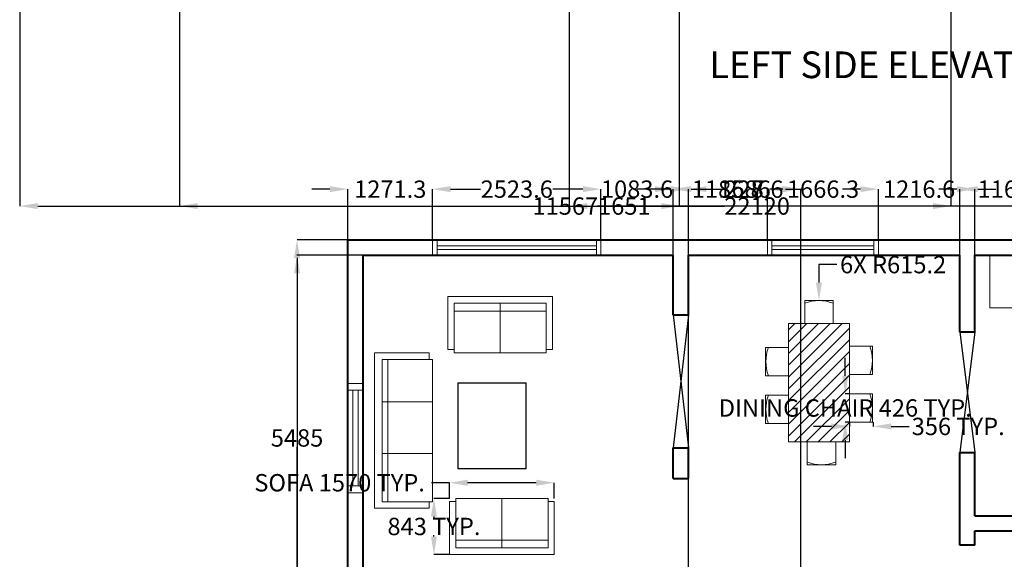
# Model space of a CAD drawing. Units: millimetres. Extents: x 23 to 3809233, y 4 to 290343.
# Tile 2 of 8: x 1893468 to 1908235, y 143728 to 151826. Entities that reach past the tile are written whole.
import ezdxf

# ---------------------------------------------------------------- set-up
doc = ezdxf.new("R2010")
doc.units = ezdxf.units.MM
doc.header["$MEASUREMENT"] = 0
for name, color, linetype, lineweight in [('A-ANNO-DIMS', 2, 'Continuous', 18), ('A-ANNO-TEXT', 7, 'Continuous', 25), ('A-DOOR', 3, 'Continuous', 25), ('A-FLOR-CASE', 8, 'Continuous', 20), ('A-FURN', 8, 'Continuous', 18), ('A-FURN-PATT', 252, 'Continuous', 13), ('A-GLAZ', 4, 'Continuous', 18), ('A-WALL', 7, 'Continuous', 40)]:
    doc.layers.add(name, color=color, linetype=linetype, lineweight=lineweight)
doc.styles.get("Standard").update_dxf_attribs({"font": 'arial.ttf'})
doc.dimstyles.get("Standard").update_dxf_attribs({"dimtxt": 260.18, "dimasz": 270.18, "dimexe": 0.18, "dimexo": 0.0625, "dimgap": 0.09, "dimtad": 0, "dimtih": 1, "dimtoh": 1, "dimdec": 0, "dimzin": 0, "dimdsep": 46, "dimtxsty": 'Standard', "dimcen": 0.09, "dimadec": 0, "dimazin": 0, "dimtfac": 1, "dimtdec": 0, "dimtofl": 0, "dimtmove": 0, "dimatfit": 3, "dimfxl": 1, "dimtolj": 1, "dimtzin": 0, "dimarcsym": 0})

# ---------------------------------------------------------------- blocks, each defined once
blk = doc.blocks.new('SOFA-TWO-SEAT')
for p, q in [((785, 743), (785, 0)), ((94, 626), (1476, 626))]:
    blk.add_line(p, q)
for points in [[(94, 743), (94, 47), (0, 47), (0, 843), (94, 843)], [(1475, 843), (94, 843)], [(94, 743), (1475, 743)], [(1475, 843), (1570, 843), (1570, 47), (1475, 47), (1475, 743)]]:
    blk.add_lwpolyline(points)
blk.add_lwpolyline([(94, 743), (1476, 743), (1476, 0), (94, 0)], close=True)
blk = doc.blocks.new('CHAIR-DINING')
blk.add_lwpolyline([(426, 0), (426, 347), (0, 347), (0, 0)])
blk.add_arc((213, -272), 615, 69.7648, 110.2352)
blk = doc.blocks.new('*D22')
at = {"layer": 'A-ANNO-DIMS', "color": 0, "lineweight": -2, "transparency": 16777216}
for p, q in [((1905849, 146482), (1905849, 146752)), ((1905912, 146212), (1905849, 146212)), ((1905912, 145786), (1905849, 145786)), ((1905849, 145516), (1905849, 145246))]:
    blk.add_line(p, q, dxfattribs=at)
at = {"layer": 'A-ANNO-DIMS', "color": 0, "transparency": 16777216}
for points in [[(1905804, 146482), (1905894, 146482), (1905849, 146212)], [(1905804, 145516), (1905894, 145516), (1905849, 145786)]]:
    blk.add_solid(points, dxfattribs=at)
at = {"layer": 'Defpoints', "color": 0, "transparency": 16777216}
for p in [(1905913, 146212), (1905849, 145786), (1905913, 145786)]:
    blk.add_point(p, dxfattribs=at)
at = {"layer": 'A-ANNO-DIMS', "color": 0, "transparency": 16777216, "insert": (1905849, 145999), "char_height": 260.18, "attachment_point": 5}
blk.add_mtext('\\A1;DINING CHAIR 426 TYP.', dxfattribs=at)
blk = doc.blocks.new('*D23')
at = {"layer": 'A-ANNO-DIMS', "color": 0, "lineweight": -2, "transparency": 16777216}
for p, q in [((1905913, 145786), (1905913, 145722)), ((1906268, 145786), (1906268, 145722)), ((1905642, 145722), (1905372, 145722)), ((1906538, 145722), (1906809, 145722))]:
    blk.add_line(p, q, dxfattribs=at)
at = {"layer": 'A-ANNO-DIMS', "color": 0, "transparency": 16777216}
for points in [[(1905642, 145767), (1905642, 145677), (1905913, 145722)], [(1906538, 145767), (1906538, 145677), (1906268, 145722)]]:
    blk.add_solid(points, dxfattribs=at)
at = {"layer": 'Defpoints', "color": 0, "transparency": 16777216}
for p in [(1905913, 145786), (1906268, 145786), (1906268, 145722)]:
    blk.add_point(p, dxfattribs=at)
at = {"layer": 'A-ANNO-DIMS', "color": 0, "transparency": 16777216, "insert": (1907543, 145722), "char_height": 260.18, "attachment_point": 5}
blk.add_mtext('\\A1;356 TYP.', dxfattribs=at)
blk = doc.blocks.new('*D24')
at = {"layer": 'A-ANNO-DIMS', "color": 0, "lineweight": -2, "transparency": 16777216}
for p, q in [((1899916, 144877), (1899646, 144877)), ((1899916, 144642), (1899916, 144878)), ((1901216, 144877), (1900186, 144877)), ((1901486, 144642), (1901486, 144878))]:
    blk.add_line(p, q, dxfattribs=at)
at = {"layer": 'A-ANNO-DIMS', "color": 0, "transparency": 16777216}
for points in [[(1900186, 144923), (1900186, 144832), (1899916, 144877)], [(1901216, 144923), (1901216, 144832), (1901486, 144877)]]:
    blk.add_solid(points, dxfattribs=at)
at = {"layer": 'Defpoints', "color": 0, "transparency": 16777216}
for p in [(1899916, 144877), (1899916, 144642), (1901486, 144642)]:
    blk.add_point(p, dxfattribs=at)
at = {"layer": 'A-ANNO-DIMS', "color": 0, "transparency": 16777216, "insert": (1898266, 144877), "char_height": 260.18, "attachment_point": 5}
blk.add_mtext('\\A1;SOFA 1570 TYP.', dxfattribs=at)
blk = doc.blocks.new('*D25')
at = {"layer": 'A-ANNO-DIMS', "color": 0, "lineweight": -2, "transparency": 16777216}
for p, q in [((1899916, 144642), (1899681, 144642)), ((1899681, 144372), (1899681, 144354)), ((1899681, 144070), (1899681, 144088)), ((1899916, 143799), (1899681, 143799))]:
    blk.add_line(p, q, dxfattribs=at)
at = {"layer": 'A-ANNO-DIMS', "color": 0, "transparency": 16777216}
for points in [[(1899636, 144372), (1899726, 144372), (1899681, 144642)], [(1899636, 144070), (1899726, 144070), (1899681, 143799)]]:
    blk.add_solid(points, dxfattribs=at)
at = {"layer": 'Defpoints', "color": 0, "transparency": 16777216}
for p in [(1899916, 144642), (1899681, 143799), (1899916, 143799)]:
    blk.add_point(p, dxfattribs=at)
at = {"layer": 'A-ANNO-DIMS', "color": 0, "transparency": 16777216, "insert": (1899681, 144221), "char_height": 260.18, "attachment_point": 5}
blk.add_mtext('\\A1;843 TYP.', dxfattribs=at)
blk = doc.blocks.new('*D49')
at = {"layer": 'A-ANNO-DIMS', "color": 0, "lineweight": -2, "transparency": 16777216}
for p, q in [((1898389.991383, 148520.288959), (1897627.373883, 148520.288959)), ((1897627.553883, 148250.108959), (1897627.553883, 141764.705112)), ((1897627.553883, 135013.262029), (1897627.553883, 141498.665876)), ((1904356.772229, 134743.082029), (1897627.373883, 134743.082029))]:
    blk.add_line(p, q, dxfattribs=at)
at = {"layer": 'A-ANNO-DIMS', "color": 0, "transparency": 16777216}
for points in [[(1897582.523883, 148250.108959), (1897672.583883, 148250.108959), (1897627.553883, 148520.288959)], [(1897582.523883, 135013.262029), (1897672.583883, 135013.262029), (1897627.553883, 134743.082029)]]:
    blk.add_solid(points, dxfattribs=at)
at = {"layer": 'Defpoints', "color": 0, "transparency": 16777216}
for p in [(1897627.553883, 148520.288959), (1898390.053883, 148520.288959), (1904356.834729, 134743.082029)]:
    blk.add_point(p, dxfattribs=at)
at = {"layer": 'A-ANNO-DIMS', "color": 0, "transparency": 16777216, "insert": (1897627.553883, 141631.685494), "char_height": 260.18, "attachment_point": 5}
blk.add_mtext('\\A1;13777', dxfattribs=at)
blk = doc.blocks.new('*D52')
at = {"layer": 'A-ANNO-DIMS', "color": 0, "lineweight": -2, "transparency": 16777216}
for p, q in [((1898619, 148292), (1897627, 148292)), ((1897628, 148022), (1897628, 145682)), ((1897628, 143076), (1897628, 145416)), ((1898619, 142806), (1897627, 142806))]:
    blk.add_line(p, q, dxfattribs=at)
at = {"layer": 'A-ANNO-DIMS', "color": 0, "transparency": 16777216}
for points in [[(1897583, 148022), (1897673, 148022), (1897628, 148292)], [(1897583, 143076), (1897673, 143076), (1897628, 142806)]]:
    blk.add_solid(points, dxfattribs=at)
at = {"layer": 'Defpoints', "color": 0, "transparency": 16777216}
for p in [(1897628, 148292), (1898619, 148292), (1898619, 142806)]:
    blk.add_point(p, dxfattribs=at)
at = {"layer": 'A-ANNO-DIMS', "color": 0, "transparency": 16777216, "insert": (1897628, 145549), "char_height": 260.2, "attachment_point": 5}
blk.add_mtext('\\A1;5485', dxfattribs=at)
blk = doc.blocks.new('*D57')
at = {"layer": 'A-ANNO-DIMS', "color": 0, "lineweight": -2, "transparency": 16777216}
for p, q in [((1898119.873883, 149282.788959), (1897849.693883, 149282.788959)), ((1898390.053883, 148520.351459), (1898390.053883, 149282.968959)), ((1899661.375825, 148520.351459), (1899661.375825, 149282.968959)), ((1899931.555825, 149282.788959), (1900201.735825, 149282.788959))]:
    blk.add_line(p, q, dxfattribs=at)
at = {"layer": 'A-ANNO-DIMS', "color": 0, "transparency": 16777216}
for points in [[(1898119.873883, 149327.818959), (1898119.873883, 149237.758959), (1898390.053883, 149282.788959)], [(1899931.555825, 149327.818959), (1899931.555825, 149237.758959), (1899661.375825, 149282.788959)]]:
    blk.add_solid(points, dxfattribs=at)
at = {"layer": 'Defpoints', "color": 0, "transparency": 16777216}
for p in [(1899661.375825, 149282.788959), (1898390.053883, 148520.288959), (1899661.375825, 148520.288959)]:
    blk.add_point(p, dxfattribs=at)
at = {"layer": 'A-ANNO-DIMS', "color": 0, "transparency": 16777216, "insert": (1899025.714854, 149282.788959), "char_height": 260.18, "attachment_point": 5}
blk.add_mtext('\\A1;1271.3', dxfattribs=at)
blk = doc.blocks.new('*D58')
at = {"layer": 'A-ANNO-DIMS', "color": 0, "lineweight": -2, "transparency": 16777216}
for p, q in [((1899661, 148520), (1899661, 149283)), ((1899932, 149283), (1900381, 149283)), ((1901915, 149283), (1901465, 149283)), ((1902185, 148520), (1902185, 149283))]:
    blk.add_line(p, q, dxfattribs=at)
at = {"layer": 'A-ANNO-DIMS', "color": 0, "transparency": 16777216}
for points in [[(1899932, 149328), (1899932, 149238), (1899661, 149283)], [(1901915, 149328), (1901915, 149238), (1902185, 149283)]]:
    blk.add_solid(points, dxfattribs=at)
at = {"layer": 'Defpoints', "color": 0, "transparency": 16777216}
for p in [(1902185, 149283), (1899661, 148520), (1902185, 148520)]:
    blk.add_point(p, dxfattribs=at)
at = {"layer": 'A-ANNO-DIMS', "color": 0, "transparency": 16777216, "insert": (1900923, 149283), "char_height": 260.2, "attachment_point": 5}
blk.add_mtext('\\A1;2523.6', dxfattribs=at)
blk = doc.blocks.new('*D59')
at = {"layer": 'A-ANNO-DIMS', "color": 0, "lineweight": -2, "transparency": 16777216}
for p, q in [((1901915, 149283), (1901645, 149283)), ((1902185, 148520), (1902185, 149283)), ((1903269, 148292), (1903269, 149283)), ((1903539, 149283), (1903809, 149283))]:
    blk.add_line(p, q, dxfattribs=at)
at = {"layer": 'A-ANNO-DIMS', "color": 0, "transparency": 16777216}
for points in [[(1901915, 149328), (1901915, 149238), (1902185, 149283)], [(1903539, 149328), (1903539, 149238), (1903269, 149283)]]:
    blk.add_solid(points, dxfattribs=at)
at = {"layer": 'Defpoints', "color": 0, "transparency": 16777216}
for p in [(1903269, 149283), (1902185, 148520), (1903269, 148292)]:
    blk.add_point(p, dxfattribs=at)
at = {"layer": 'A-ANNO-DIMS', "color": 0, "transparency": 16777216, "insert": (1902727, 149283), "char_height": 260.2, "attachment_point": 5}
blk.add_mtext('\\A1;1083.6', dxfattribs=at)
blk = doc.blocks.new('*D60')
at = {"layer": 'A-ANNO-DIMS', "color": 0, "lineweight": -2, "transparency": 16777216}
for p, q in [((1902998, 149283), (1902728, 149283)), ((1903269, 148292), (1903269, 149283)), ((1903497, 148292), (1903497, 149283)), ((1903767, 149283), (1904038, 149283))]:
    blk.add_line(p, q, dxfattribs=at)
at = {"layer": 'A-ANNO-DIMS', "color": 0, "transparency": 16777216}
for points in [[(1902998, 149328), (1902998, 149238), (1903269, 149283)], [(1903767, 149328), (1903767, 149238), (1903497, 149283)]]:
    blk.add_solid(points, dxfattribs=at)
at = {"layer": 'Defpoints', "color": 0, "transparency": 16777216}
for p in [(1903497, 149283), (1903269, 148292), (1903497, 148292)]:
    blk.add_point(p, dxfattribs=at)
at = {"layer": 'A-ANNO-DIMS', "color": 0, "transparency": 16777216, "insert": (1904479, 149283), "char_height": 260.2, "attachment_point": 5}
blk.add_mtext('\\A1;228.6', dxfattribs=at)
blk = doc.blocks.new('*D61')
at = {"layer": 'A-ANNO-DIMS', "color": 0, "lineweight": -2, "transparency": 16777216}
for p, q in [((1903227, 149283), (1902957, 149283)), ((1903497, 148292), (1903497, 149283)), ((1904683, 148520), (1904683, 149283)), ((1904953, 149283), (1905223, 149283))]:
    blk.add_line(p, q, dxfattribs=at)
at = {"layer": 'A-ANNO-DIMS', "color": 0, "transparency": 16777216}
for points in [[(1903227, 149328), (1903227, 149238), (1903497, 149283)], [(1904953, 149328), (1904953, 149238), (1904683, 149283)]]:
    blk.add_solid(points, dxfattribs=at)
at = {"layer": 'Defpoints', "color": 0, "transparency": 16777216}
for p in [(1904683, 149283), (1904683, 148520), (1903497, 148292)]:
    blk.add_point(p, dxfattribs=at)
at = {"layer": 'A-ANNO-DIMS', "color": 0, "transparency": 16777216, "insert": (1904090, 149283), "char_height": 260.2, "attachment_point": 5}
blk.add_mtext('\\A1;1185.7', dxfattribs=at)
blk = doc.blocks.new('*D62')
at = {"layer": 'A-ANNO-DIMS', "color": 0, "lineweight": -2, "transparency": 16777216}
for p, q in [((1904683, 148520), (1904683, 149283)), ((1904953, 149283), (1904988, 149283)), ((1906079, 149283), (1906044, 149283)), ((1906349, 148520), (1906349, 149283))]:
    blk.add_line(p, q, dxfattribs=at)
at = {"layer": 'A-ANNO-DIMS', "color": 0, "transparency": 16777216}
for points in [[(1904953, 149328), (1904953, 149238), (1904683, 149283)], [(1906079, 149328), (1906079, 149238), (1906349, 149283)]]:
    blk.add_solid(points, dxfattribs=at)
at = {"layer": 'Defpoints', "color": 0, "transparency": 16777216}
for p in [(1906349, 149283), (1904683, 148520), (1906349, 148520)]:
    blk.add_point(p, dxfattribs=at)
at = {"layer": 'A-ANNO-DIMS', "color": 0, "transparency": 16777216, "insert": (1905516, 149283), "char_height": 260.2, "attachment_point": 5}
blk.add_mtext('\\A1;1666.3', dxfattribs=at)
blk = doc.blocks.new('*D63')
at = {"layer": 'A-ANNO-DIMS', "color": 0, "lineweight": -2, "transparency": 16777216}
for p, q in [((1906079, 149283), (1905809, 149283)), ((1906349, 148520), (1906349, 149283)), ((1907566, 148292), (1907566, 149283)), ((1907836, 149283), (1908106, 149283))]:
    blk.add_line(p, q, dxfattribs=at)
at = {"layer": 'A-ANNO-DIMS', "color": 0, "transparency": 16777216}
for points in [[(1906079, 149328), (1906079, 149238), (1906349, 149283)], [(1907836, 149328), (1907836, 149238), (1907566, 149283)]]:
    blk.add_solid(points, dxfattribs=at)
at = {"layer": 'Defpoints', "color": 0, "transparency": 16777216}
for p in [(1907566, 149283), (1906349, 148520), (1907566, 148292)]:
    blk.add_point(p, dxfattribs=at)
at = {"layer": 'A-ANNO-DIMS', "color": 0, "transparency": 16777216, "insert": (1906957, 149283), "char_height": 260.2, "attachment_point": 5}
blk.add_mtext('\\A1;1216.6', dxfattribs=at)
blk = doc.blocks.new('*D64')
at = {"layer": 'A-ANNO-DIMS', "color": 0, "lineweight": -2, "transparency": 16777216}
for p, q in [((1907524.135363, 149282.788959), (1907253.955363, 149282.788959)), ((1907794.315363, 148291.751459), (1907794.315363, 149282.968959)), ((1908956.509231, 148520.351459), (1908956.509231, 149282.968959)), ((1909226.689231, 149282.788959), (1909496.869231, 149282.788959))]:
    blk.add_line(p, q, dxfattribs=at)
at = {"layer": 'A-ANNO-DIMS', "color": 0, "transparency": 16777216}
for points in [[(1907524.135363, 149327.818959), (1907524.135363, 149237.758959), (1907794.315363, 149282.788959)], [(1909226.689231, 149327.818959), (1909226.689231, 149237.758959), (1908956.509231, 149282.788959)]]:
    blk.add_solid(points, dxfattribs=at)
at = {"layer": 'Defpoints', "color": 0, "transparency": 16777216}
for p in [(1908956.509231, 149282.788959), (1908956.509231, 148520.288959), (1907794.315363, 148291.688959)]:
    blk.add_point(p, dxfattribs=at)
at = {"layer": 'A-ANNO-DIMS', "color": 0, "transparency": 16777216, "insert": (1908375.412297, 149282.788959), "char_height": 260.18, "attachment_point": 5}
blk.add_mtext('\\A1;1162.2', dxfattribs=at)
blk = doc.blocks.new('*D70')
at = {"layer": 'A-ANNO-DIMS', "color": 0, "lineweight": -2, "transparency": 16777216}
for p, q in [((1903497, 142880), (1903497, 149283)), ((1903767, 149283), (1903964, 149283)), ((1904913, 149283), (1904716, 149283)), ((1905183, 142880), (1905183, 149283))]:
    blk.add_line(p, q, dxfattribs=at)
at = {"layer": 'A-ANNO-DIMS', "color": 0, "transparency": 16777216}
for points in [[(1903767, 149328), (1903767, 149238), (1903497, 149283)], [(1904913, 149328), (1904913, 149238), (1905183, 149283)]]:
    blk.add_solid(points, dxfattribs=at)
at = {"layer": 'Defpoints', "color": 0, "transparency": 16777216}
for p in [(1905183, 149283), (1903497, 142880), (1905183, 142880)]:
    blk.add_point(p, dxfattribs=at)
at = {"layer": 'A-ANNO-DIMS', "color": 0, "transparency": 16777216, "insert": (1904340, 149283), "char_height": 260.2, "attachment_point": 5}
blk.add_mtext('\\A1;1686', dxfattribs=at)
blk = doc.blocks.new('*D80')
at = {"layer": 'A-ANNO-DIMS', "color": 0, "lineweight": -2, "transparency": 16777216}
for p, q in [((1893468, 163690), (1893468, 149029)), ((1915588, 152264), (1915588, 149029)), ((1893739, 149029), (1904037, 149029)), ((1915318, 149029), (1905020, 149029))]:
    blk.add_line(p, q, dxfattribs=at)
at = {"layer": 'A-ANNO-DIMS', "color": 0, "transparency": 16777216}
for points in [[(1893739, 149074), (1893739, 148984), (1893468, 149029)], [(1915318, 149074), (1915318, 148984), (1915588, 149029)]]:
    blk.add_solid(points, dxfattribs=at)
at = {"layer": 'Defpoints', "color": 0, "transparency": 16777216}
for p in [(1893468, 163690), (1915588, 152265), (1915588, 149029)]:
    blk.add_point(p, dxfattribs=at)
at = {"layer": 'A-ANNO-DIMS', "color": 0, "transparency": 16777216, "insert": (1904528, 149029), "char_height": 260.2, "attachment_point": 5}
blk.add_mtext('\\A1;22120', dxfattribs=at)
blk = doc.blocks.new('*D82')
at = {"layer": 'A-ANNO-DIMS', "color": 0, "lineweight": -2, "transparency": 16777216}
for p, q in [((1895867, 152264), (1895867, 149029)), ((1907434, 152264), (1907434, 149029)), ((1896137, 149029), (1901173, 149029)), ((1907164, 149029), (1902128, 149029))]:
    blk.add_line(p, q, dxfattribs=at)
at = {"layer": 'A-ANNO-DIMS', "color": 0, "transparency": 16777216}
for points in [[(1896137, 149074), (1896137, 148984), (1895867, 149029)], [(1907164, 149074), (1907164, 148984), (1907434, 149029)]]:
    blk.add_solid(points, dxfattribs=at)
at = {"layer": 'Defpoints', "color": 0, "transparency": 16777216}
for p in [(1895867, 152265), (1907434, 152265), (1907434, 149029)]:
    blk.add_point(p, dxfattribs=at)
at = {"layer": 'A-ANNO-DIMS', "color": 0, "transparency": 16777216, "insert": (1901651, 149029), "char_height": 260.2, "attachment_point": 5}
blk.add_mtext('\\A1;11567', dxfattribs=at)
blk = doc.blocks.new('*D85')
at = {"layer": 'A-ANNO-DIMS', "color": 0, "lineweight": -2, "transparency": 16777216}
for p, q in [((1901710, 158781), (1901710, 149029)), ((1903361, 158781), (1903361, 149029)), ((1901980, 149029), (1902184, 149029)), ((1903091, 149029), (1902887, 149029))]:
    blk.add_line(p, q, dxfattribs=at)
at = {"layer": 'A-ANNO-DIMS', "color": 0, "transparency": 16777216}
for points in [[(1901980, 149074), (1901980, 148984), (1901710, 149029)], [(1903091, 149074), (1903091, 148984), (1903361, 149029)]]:
    blk.add_solid(points, dxfattribs=at)
at = {"layer": 'Defpoints', "color": 0, "transparency": 16777216}
for p in [(1901710, 158781), (1903361, 158781), (1903361, 149029)]:
    blk.add_point(p, dxfattribs=at)
at = {"layer": 'A-ANNO-DIMS', "color": 0, "transparency": 16777216, "insert": (1902536, 149029), "char_height": 260.2, "attachment_point": 5}
blk.add_mtext('\\A1;1651', dxfattribs=at)
blk = doc.blocks.new('*D126')
at = {"layer": 'A-ANNO-DIMS', "color": 0, "lineweight": -2, "transparency": 16777216}
for p, q in [((1905725, 148150), (1905455, 148150)), ((1905455, 148150), (1905455, 147880)), ((1905455, 146995), (1905455, 146995)), ((1905455, 146995), (1905455, 146995))]:
    blk.add_line(p, q, dxfattribs=at)
at = {"layer": 'A-ANNO-DIMS', "color": 0, "transparency": 16777216}
blk.add_solid([(1905410, 147880), (1905500, 147880), (1905455, 147610)], dxfattribs=at)
at = {"layer": 'Defpoints', "color": 0, "transparency": 16777216}
for p in [(1905455, 147610), (1905455, 146995)]:
    blk.add_point(p, dxfattribs=at)
at = {"layer": 'A-ANNO-DIMS', "color": 0, "transparency": 16777216, "insert": (1906567, 148150), "char_height": 260.18, "attachment_point": 5}
blk.add_mtext('\\A1;6X R615.2', dxfattribs=at)

msp = doc.modelspace()

# ---------------------------------------------------------------- hatches: boundary and pattern name
at = {"layer": 'A-FURN-PATT'}
h = msp.add_hatch(dxfattribs=at)
h.set_pattern_fill('ANSI31', color=256, scale=1001.108828)
h.set_pattern_definition([(45, (-1834512.67, -141903.28), (-88.486355, 88.486355), [])])
h.paths.add_polyline_path([(1905911.064, 147267.073), (1904998.148, 147267.073), (1904998.148, 145490.669), (1905911.064, 145490.669)])

# ---------------------------------------------------------------- linework, layer by layer
at = {"layer": 'A-DOOR'}
for p, q in [((1903268.565, 147398.847), (1903497.165, 145399.614)), ((1903497.165, 147398.847), (1903268.565, 145399.614)), ((1907565.715, 147142.642), (1907794.315, 145331.486)), ((1907794.315, 147142.642), (1907565.715, 145331.486))]:
    msp.add_line(p, q, dxfattribs=at)
at = {"layer": 'A-FLOR-CASE'}
for p, q in [((1908018.892, 148291.689), (1908018.892, 147503.249)), ((1908018.892, 147503.249), (1910929.729, 147503.249))]:
    msp.add_line(p, q, dxfattribs=at)
at = {"layer": 'A-FURN'}
for p, q in [((1898991.206, 146728.547), (1898991.206, 144592.7)), ((1898906.834, 146089.094), (1899660.017, 146089.094)), ((1898906.834, 145314.243), (1899660.017, 145314.243))]:
    msp.add_line(p, q, dxfattribs=at)
for points in [[(1904998.148, 147267.073), (1905911.064, 147267.073), (1905911.064, 145490.669), (1904998.148, 145490.669)], [(1899660.017, 146728.547), (1898906.834, 146728.547), (1898906.834, 144592.7), (1899660.017, 144592.7)], [(1900038.698, 146376.334), (1901064.866, 146376.334), (1901064.866, 145087.893), (1900038.698, 145087.893)], [(1900043.698, 146371.334), (1901059.866, 146371.334), (1901059.866, 145092.893), (1900043.698, 145092.893)]]:
    msp.add_lwpolyline(points, close=True, dxfattribs=at)
for points in [[(1898906.834, 146728.547), (1899609.754, 146728.547), (1899609.754, 146824.515), (1898790.034, 146824.515), (1898790.034, 146728.547)], [(1898790.034, 146728.547), (1898790.034, 144590.856)], [(1898906.834, 144590.856), (1898906.834, 146728.547)], [(1898790.034, 144590.856), (1898790.034, 144494.888), (1899609.754, 144494.888), (1899609.754, 144590.856), (1898906.834, 144590.856)]]:
    msp.add_lwpolyline(points, dxfattribs=at)
at = {"layer": 'A-GLAZ'}
for p, q in [((1899661.376, 148520.289), (1899661.376, 148291.689)), ((1899728.787, 148520.289), (1899728.787, 148291.689)), ((1899728.787, 148434.405), (1902119.979, 148434.405)), ((1902119.979, 148520.289), (1902119.979, 148291.689)), ((1902184.948, 148520.289), (1902184.948, 148291.689)), ((1904682.851, 148520.289), (1904682.851, 148291.689)), ((1904750.449, 148520.289), (1904750.449, 148291.689)), ((1904750.449, 148430.572), (1906279.934, 148430.572)), ((1906279.934, 148520.289), (1906279.934, 148291.689)), ((1906349.105, 148520.289), (1906349.105, 148291.689)), ((1899728.787, 148379.313), (1902119.979, 148379.313)), ((1904750.449, 148379.503), (1906279.934, 148379.503)), ((1898390.054, 146365.369), (1898618.654, 146365.369)), ((1898390.054, 146266.357), (1898618.654, 146266.357)), ((1898462.596, 146266.357), (1898462.596, 144832.424)), ((1898544.24, 146266.357), (1898544.24, 144832.424)), ((1898390.054, 144832.424), (1898618.654, 144832.424)), ((1898390.054, 144726.679), (1898618.654, 144726.679)), ((1898544.24, 144832.424), (1898544.24, 144832.424))]:
    msp.add_line(p, q, dxfattribs=at)
at = {"layer": 'A-WALL'}
for p, q in [((1898390.054, 148520.289), (1912047.254, 148520.289)), ((1898390.054, 135763.089), (1898390.054, 148520.289)), ((1898618.654, 148291.689), (1903268.565, 148291.689)), ((1898618.654, 142806.221), (1898618.654, 148291.689)), ((1903268.565, 147398.847), (1903268.565, 148291.689)), ((1903497.165, 148291.689), (1907565.715, 148291.689)), ((1903497.165, 147398.847), (1903497.165, 148291.689)), ((1907565.715, 147142.642), (1907565.715, 148291.689)), ((1907794.315, 148291.689), (1911818.654, 148291.689)), ((1907794.315, 147142.642), (1907794.315, 148291.689)), ((1903268.565, 147398.847), (1903497.165, 147398.847)), ((1907565.715, 147142.642), (1907794.315, 147142.642)), ((1903268.565, 145399.614), (1903497.165, 145399.614)), ((1903268.565, 144943.006), (1903268.565, 145399.614)), ((1903497.165, 144943.006), (1903497.165, 145399.614)), ((1907565.715, 145331.486), (1907794.315, 145331.486)), ((1907565.715, 143941.277), (1907565.715, 145331.486)), ((1907794.315, 144382.478), (1907794.315, 145331.486)), ((1903268.565, 144943.006), (1903497.165, 144943.006)), ((1907794.315, 144382.478), (1909015.346, 144382.478)), ((1907794.315, 143941.277), (1907794.315, 144153.878)), ((1907794.315, 144153.878), (1909015.346, 144153.878)), ((1907794.315, 143941.277), (1907565.715, 143941.277))]:
    msp.add_line(p, q, dxfattribs=at)

# ---------------------------------------------------------------- block references
at = {"layer": 'A-FURN'}
for name, p in [('SOFA-TWO-SEAT', (1899887.775, 146827.63)), ('CHAIR-DINING', (1905241.829, 147267.073))]:
    msp.add_blockref(name, p, dxfattribs=at)
for name, p, rotation in [('CHAIR-DINING', (1905912.77, 146926.558), 269.9999999999404), ('CHAIR-DINING', (1905002.137, 146481.78), 89.99999999994041), ('CHAIR-DINING', (1905002.137, 145764.843), 89.99999999994041), ('CHAIR-DINING', (1905912.516, 146211.752), 269.9999999999285), ('CHAIR-DINING', (1905705.715, 145490.669), 180), ('SOFA-TWO-SEAT', (1901485.754, 144642.051), 180)]:
    msp.add_blockref(name, p, dxfattribs=dict(at, rotation=rotation))

# ---------------------------------------------------------------- texts
at = {"layer": 'A-ANNO-TEXT', "insert": (1903808.34, 151348.696), "char_height": 400, "attachment_point": 1}
msp.add_mtext_dynamic_manual_height_columns('LEFT SIDE ELEVATION', width=8410.77875, gutter_width=1, heights=[307.465], dxfattribs=at)

# ---------------------------------------------------------------- dimensions: what is measured, and where the dimension line sits
at = {"layer": 'A-ANNO-DIMS'}
for base, p1, p2, override, picture, middle in [((1915588.32, 149029.101), (1893468.322, 163689.971), (1915588.32, 152264.531), {"dimdec": 0, "dimlfac": 1, "dimrnd": 0, "dimzin": 0, "dimdsep": 46, "dimlunit": 2}, '*D80', (1904528.321, 149029.101)), ((1903361.093, 149029.101), (1901710.076, 158780.768), (1903361.093, 158780.768), {"dimdec": 0, "dimlfac": 1, "dimrnd": 0, "dimzin": 0, "dimdsep": 46, "dimlunit": 2}, '*D85', (1902535.585, 149029.101)), ((1907434.445, 149029.101), (1895867.197, 152264.531), (1907434.445, 152264.531), {"dimdec": 0, "dimlfac": 1, "dimrnd": 0, "dimzin": 0, "dimdsep": 46, "dimlunit": 2}, '*D82', (1901650.821, 149029.101)), ((1899661.376, 149282.789), (1898390.054, 148520.289), (1899661.376, 148520.289), {"dimdec": 1, "dimlfac": 1, "dimrnd": 0, "dimzin": 0, "dimdsep": 46, "dimlunit": 2}, '*D57', (1899025.715, 149282.789)), ((1902184.948, 149282.789), (1899661.376, 148520.289), (1902184.948, 148520.289), {"dimdec": 1, "dimlfac": 1, "dimrnd": 0, "dimzin": 0, "dimdsep": 46, "dimlunit": 2}, '*D58', (1900923.162, 149282.789)), ((1903268.565, 149282.789), (1902184.948, 148520.289), (1903268.565, 148291.689), {"dimdec": 1, "dimlfac": 1, "dimrnd": 0, "dimzin": 0, "dimdsep": 46, "dimlunit": 2}, '*D59', (1902726.756, 149282.789)), ((1903497.165, 149282.789), (1903268.565, 148291.689), (1903497.165, 148291.689), {"dimdec": 1, "dimlfac": 1, "dimrnd": 0, "dimzin": 0, "dimdsep": 46, "dimlunit": 2}, '*D60', (1904478.732, 149282.789)), ((1904682.851, 149282.789), (1903497.165, 148291.689), (1904682.851, 148520.289), {"dimdec": 1, "dimlfac": 1, "dimrnd": 0, "dimzin": 0, "dimdsep": 46, "dimlunit": 2}, '*D61', (1904090.008, 149282.789)), ((1905183.132, 149282.789), (1903497.165, 142879.905), (1905183.132, 142879.905), {"dimdec": 0, "dimlfac": 1, "dimrnd": 0, "dimzin": 0, "dimdsep": 46, "dimlunit": 2}, '*D70', (1904340.149, 149282.789)), ((1906349.105, 149282.789), (1904682.851, 148520.289), (1906349.105, 148520.289), {"dimdec": 1, "dimlfac": 1, "dimrnd": 0, "dimzin": 0, "dimdsep": 46, "dimlunit": 2}, '*D62', (1905515.978, 149282.789)), ((1907565.715, 149282.789), (1906349.105, 148520.289), (1907565.715, 148291.689), {"dimdec": 1, "dimlfac": 1, "dimrnd": 0, "dimzin": 0, "dimdsep": 46, "dimlunit": 2}, '*D63', (1906957.41, 149282.789)), ((1908956.509, 149282.789), (1907794.315, 148291.689), (1908956.509, 148520.289), {"dimdec": 1, "dimlfac": 1, "dimrnd": 0, "dimzin": 0, "dimdsep": 46, "dimlunit": 2}, '*D64', (1908375.412, 149282.789))]:
    dim = msp.add_linear_dim(base=base, p1=p1, p2=p2, dimstyle='Standard', override=override, dxfattribs=at)
    dim.commit()
    dim.dimension.update_dxf_attribs({"geometry": picture, "text_midpoint": middle})
for base, p1, p2, picture, middle in [((1897627.554, 148520.289), (1904356.835, 134743.082), (1898390.054, 148520.289), '*D49', (1897627.554, 141631.685)), ((1897627.554, 148291.689), (1898618.654, 142806.221), (1898618.654, 148291.689), '*D52', (1897627.554, 145548.955))]:
    dim = msp.add_linear_dim(base=base, p1=p1, p2=p2, angle=90, dimstyle='Standard', override={"dimdec": 0, "dimlfac": 1, "dimrnd": 0, "dimzin": 0, "dimdsep": 46, "dimlunit": 2}, dxfattribs=at)
    dim.commit()
    dim.dimension.update_dxf_attribs({"geometry": picture, "text_midpoint": middle})
dim = msp.add_radius_dim(center=(1905454.606, 146994.889), mpoint=(1905454.606, 147610.073), text='6X <>', dimstyle='Standard', override={"dimdec": 1, "dimlfac": 1, "dimrnd": 0, "dimzin": 0, "dimdsep": 46, "dimlunit": 2}, dxfattribs=at)
dim.commit()
dim.dimension.update_dxf_attribs({"geometry": '*D126', "text_midpoint": (1906567.266, 148150.433)})
for base, p1, p2, angle, text, picture, middle in [((1905848.683, 145786.198), (1905912.516, 146211.751), (1905912.516, 145786.198), 270, 'DINING CHAIR <> TYP.', '*D22', (1905848.683, 145998.975)), ((1899916.184, 144877.487), (1901485.754, 144642.051), (1899916.184, 144642.051), 180, 'SOFA <> TYP.', '*D24', (1898265.86, 144877.487)), ((1899680.749, 143799.491), (1899916.184, 144642.051), (1899916.184, 143799.491), 270, '<> TYP.', '*D25', (1899680.749, 144220.771))]:
    dim = msp.add_linear_dim(base=base, p1=p1, p2=p2, angle=angle, text=text, dimstyle='Standard', override={"dimdec": 0, "dimlfac": 1, "dimrnd": 0, "dimzin": 0, "dimdsep": 46, "dimlunit": 2}, dxfattribs=at)
    dim.commit()
    dim.dimension.update_dxf_attribs({"geometry": picture, "text_midpoint": middle})
dim = msp.add_linear_dim(base=(1906268.172, 145722.366), p1=(1905912.516, 145786.198), p2=(1906268.172, 145786.198), text='<> TYP.', dimstyle='Standard', override={"dimdec": 0, "dimlfac": 1, "dimrnd": 0, "dimzin": 0, "dimdsep": 46, "dimlunit": 2}, dxfattribs=at)
dim.commit()
dim.dimension.update_dxf_attribs({"geometry": '*D23', "text_midpoint": (1907542.841, 145722.366)})

doc.saveas('drawing.dxf')
